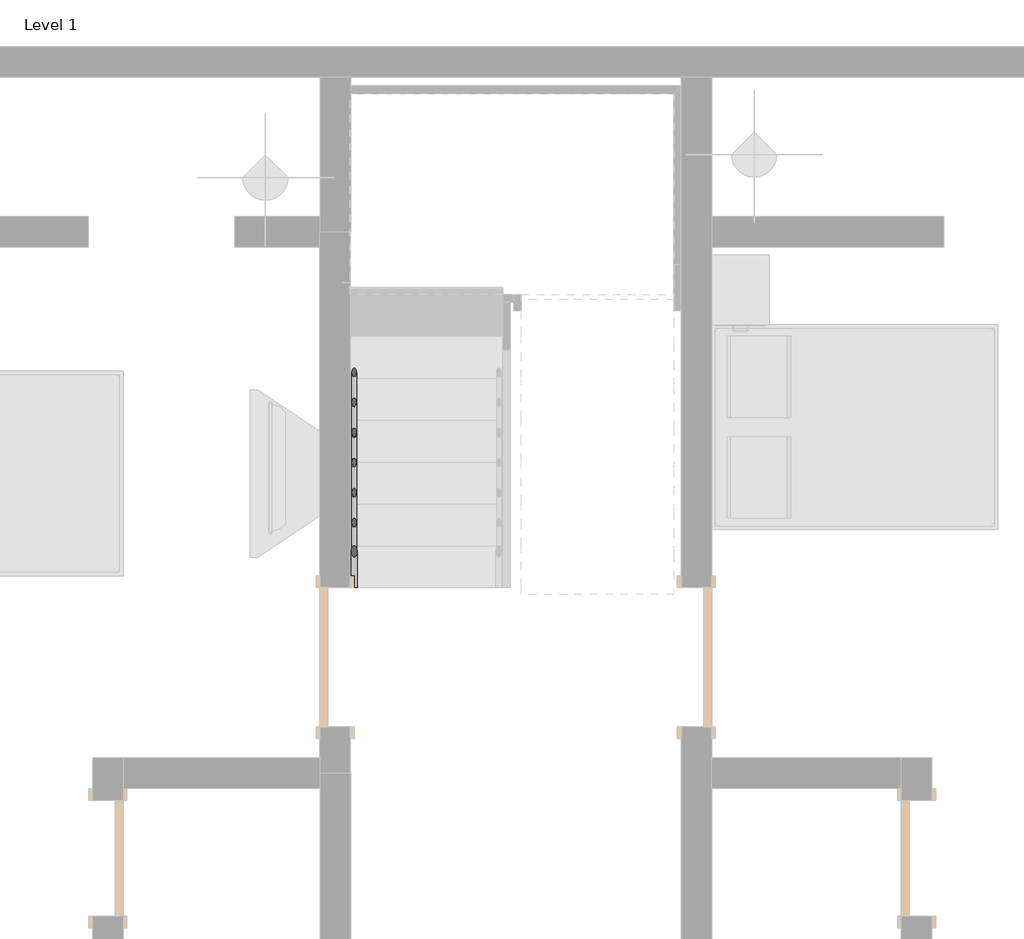
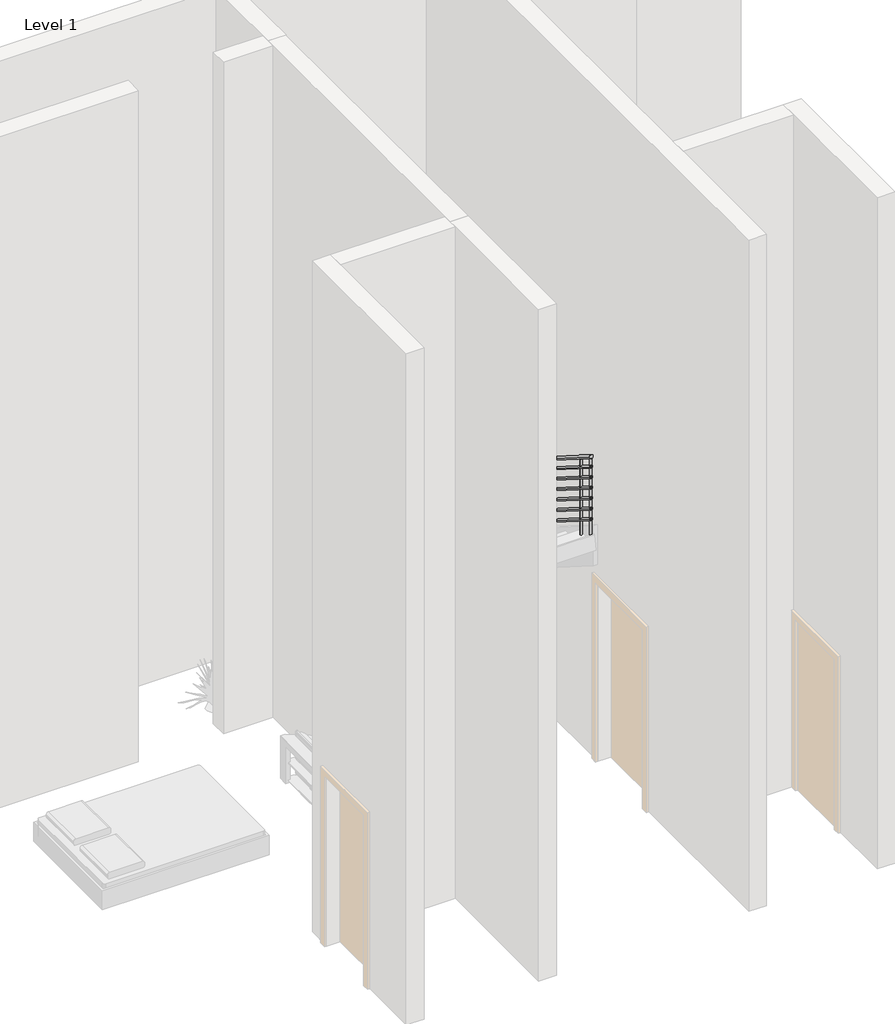
# One storey, part 3 of 4: 1 railing.
"""IFC4 building model written with IfcOpenShell, lengths in millimetres."""

from ifc_helpers import new_model, si_unit, point, frame, frame_2d, origin, place, context, project, spatial, circle_curve, ellipse_curve, trimmed, segment, composite_curve, outline, extrude, element, save
from ifc_brep_helpers import plane_surface, cylinder_surface, advanced_brep

model = new_model("IFC4")

# Units and contexts
model_context = context("Model", 3, world=origin())
ifc_project = project(units=[si_unit("LENGTHUNIT", "METRE", prefix="MILLI")], contexts=[model_context])

# Site, building, storey
site = spatial("IfcSite", under=ifc_project)
building = spatial("IfcBuilding", under=site)
storey = spatial("IfcBuildingStorey", under=building, Name="Level 1", Elevation=0.0)

# Railing
placement = place(None, origin())
element("IfcRailing", 1, ObjectType="900mm Pipe", at=placement, inside=storey, context=model_context, shape_type="SolidModel", body=[
    advanced_brep(
    [(-4517.5197318, 8898.7482221, 1050.2491997), (-4557.5197318, 8898.7482221, 1050.2491997), (-4517.5197318, 10829.5416751, 2271.3043478), (-4557.5197318, 10829.5416751, 2271.3043478), (-4517.5197318, 12099.1482221, 2271.3043478), (-4557.5197318, 12139.1482221, 2271.3043478), (-2485.6681693, 12099.1482221, 2271.3043478), (-2445.6681693, 12139.1482221, 2271.3043478), (-2485.6681693, 11092.9547691, 2271.3043478), (-2445.6681693, 11092.9547691, 2271.3043478), (-2485.6681693, 8898.7482221, 3658.9448519), (-2445.6681693, 8898.7482221, 3658.9448519)],
    [
        (0, 1, ellipse_curve(frame((-4537.5197318, 8898.7482221, 1050.2491997), z_axis=(0.0, -1.0, 0.0), x_axis=(0.0, 0.0, -1.0)), 23.6638438, 20.0)),
        (1, 0, ellipse_curve(frame((-4537.5197318, 8898.7482221, 1050.2491997), z_axis=(0.0, -1.0, 0.0), x_axis=(0.0, 0.0, -1.0)), 23.6638438, 20.0)),
        (0, 2),
        (2, 3, ellipse_curve(frame((-4537.5197318, 10829.5416751, 2271.3043478), z_axis=(0.0, -0.9605132043335073, -0.2782344053149759), x_axis=(0.0, 0.2782344053149766, -0.960513204333507)), 20.822202, 20.0)),
        (3, 1),
        (3, 2, ellipse_curve(frame((-4537.5197318, 10829.5416751, 2271.3043478), z_axis=(0.0, -0.9605132043335073, -0.2782344053149759), x_axis=(0.0, 0.2782344053149766, -0.960513204333507)), 20.822202, 20.0)),
        (2, 4),
        (4, 5, ellipse_curve(frame((-4537.5197318, 12119.1482221, 2271.3043478), z_axis=(-0.7071067811865482, -0.7071067811865468, 0.0), x_axis=(0.7071067811865468, -0.7071067811865482, 0.0)), 28.2842712, 20.0)),
        (5, 3),
        (5, 4, ellipse_curve(frame((-4537.5197318, 12119.1482221, 2271.3043478), z_axis=(-0.7071067811865482, -0.7071067811865468, 0.0), x_axis=(0.7071067811865468, -0.7071067811865482, 0.0)), 28.2842712, 20.0)),
        (4, 6),
        (6, 7, ellipse_curve(frame((-2465.6681693, 12119.1482221, 2271.3043478), z_axis=(-0.7071067811865469, 0.7071067811865481, 0.0), x_axis=(-0.7071067811865481, -0.7071067811865469, 0.0)), 28.2842712, 20.0)),
        (7, 5),
        (7, 6, ellipse_curve(frame((-2465.6681693, 12119.1482221, 2271.3043478), z_axis=(-0.7071067811865469, 0.7071067811865481, 0.0), x_axis=(-0.7071067811865481, -0.7071067811865469, 0.0)), 28.2842712, 20.0)),
        (6, 8),
        (8, 9, ellipse_curve(frame((-2465.6681693, 11092.9547691, 2271.3043478), z_axis=(0.0, 0.9605132043335073, -0.2782344053149755), x_axis=(0.0, 0.27823440531497573, 0.9605132043335072)), 20.822202, 20.0)),
        (9, 7),
        (9, 8, ellipse_curve(frame((-2465.6681693, 11092.9547691, 2271.3043478), z_axis=(0.0, 0.9605132043335073, -0.2782344053149755), x_axis=(0.0, 0.27823440531497573, 0.9605132043335072)), 20.822202, 20.0)),
        (10, 11, ellipse_curve(frame((-2465.6681693, 8898.7482221, 3658.9448519), z_axis=(0.0, -1.0, 0.0), x_axis=(0.0, 0.0, -1.0)), 23.6638438, 20.0)),
        (11, 10, ellipse_curve(frame((-2465.6681693, 8898.7482221, 3658.9448519), z_axis=(0.0, -1.0, 0.0), x_axis=(0.0, 0.0, -1.0)), 23.6638438, 20.0)),
        (8, 10),
        (11, 9),
    ],
    [
        plane_surface(frame((-4537.5197318, 8898.7482221, 1073.9130435), z_axis=(0.0, -1.0, 0.0), x_axis=(0.0, 0.0, 1.0))),
        cylinder_surface(frame((-4537.5197318, 8909.4381349, 1057.0096189), z_axis=(0.0, -0.8451712313980435, -0.5344956404098306), x_axis=(-1.0, 0.0, 0.0)), 20.0),
        cylinder_surface(frame((-4537.5197318, 10823.7482221, 2271.3043478), z_axis=(0.0, -1.0, 0.0), x_axis=(-1.0, 0.0, 0.0)), 20.0),
        cylinder_surface(frame((-4537.5197318, 12119.1482221, 2271.3043478), z_axis=(-1.0, 0.0, 0.0), x_axis=(0.0, 1.0, 0.0)), 20.0),
        cylinder_surface(frame((-2465.6681693, 12119.1482221, 2271.3043478), z_axis=(0.0, 1.0, 0.0), x_axis=(1.0, 0.0, 0.0)), 20.0),
        plane_surface(frame((-2465.6681693, 8898.7482221, 3682.6086957), z_axis=(0.0, -1.0, 0.0), x_axis=(0.0, 0.0, -1.0))),
        cylinder_surface(frame((-2465.6681693, 11088.0583093, 2274.4009232), z_axis=(0.0, 0.8451712313980438, -0.53449564040983), x_axis=(1.0, 0.0, 0.0)), 20.0),
    ],
    [
        (0, [[1, 2]]),
        (1, [[-1, 3, 4, 5]]),
        (1, [[-2, -5, 6, -3]]),
        (2, [[-4, 7, 8, 9]]),
        (2, [[-6, -9, 10, -7]]),
        (3, [[-8, 11, 12, 13]]),
        (3, [[-10, -13, 14, -11]]),
        (4, [[-12, 15, 16, 17]]),
        (4, [[-14, -17, 18, -15]]),
        (5, [[19, 20]]),
        (6, [[-16, 21, -20, 22]]),
        (6, [[-18, -22, -19, -21]]),
    ],
),
    advanced_brep(
    [(-4522.5197318, 8898.7482221, 931.1651606), (-4552.5197318, 8898.7482221, 931.1651606), (-4522.5197318, 10828.0933118, 2151.3043478), (-4552.5197318, 10828.0933118, 2151.3043478), (-4522.5197318, 12104.1482221, 2151.3043478), (-4552.5197318, 12134.1482221, 2151.3043478), (-2480.6681693, 12104.1482221, 2151.3043478), (-2450.6681693, 12134.1482221, 2151.3043478), (-2480.6681693, 11094.4031323, 2151.3043478), (-2450.6681693, 11094.4031323, 2151.3043478), (-2480.6681693, 8898.7482221, 3539.8608128), (-2450.6681693, 8898.7482221, 3539.8608128)],
    [
        (0, 1, ellipse_curve(frame((-4537.5197318, 8898.7482221, 931.1651606), z_axis=(0.0, -1.0, 0.0), x_axis=(0.0, 0.0, -1.0)), 17.7478828, 15.0)),
        (1, 0, ellipse_curve(frame((-4537.5197318, 8898.7482221, 931.1651606), z_axis=(0.0, -1.0, 0.0), x_axis=(0.0, 0.0, -1.0)), 17.7478828, 15.0)),
        (0, 2),
        (2, 3, ellipse_curve(frame((-4537.5197318, 10828.0933118, 2151.3043478), z_axis=(0.0, -0.9605132043335073, -0.2782344053149759), x_axis=(0.0, 0.2782344053149766, -0.960513204333507)), 15.6166515, 15.0)),
        (3, 1),
        (3, 2, ellipse_curve(frame((-4537.5197318, 10828.0933118, 2151.3043478), z_axis=(0.0, -0.9605132043335073, -0.2782344053149759), x_axis=(0.0, 0.2782344053149766, -0.960513204333507)), 15.6166515, 15.0)),
        (2, 4),
        (4, 5, ellipse_curve(frame((-4537.5197318, 12119.1482221, 2151.3043478), z_axis=(-0.7071067811865482, -0.7071067811865468, 0.0), x_axis=(0.7071067811865468, -0.7071067811865482, 0.0)), 21.2132034, 15.0)),
        (5, 3),
        (5, 4, ellipse_curve(frame((-4537.5197318, 12119.1482221, 2151.3043478), z_axis=(-0.7071067811865482, -0.7071067811865468, 0.0), x_axis=(0.7071067811865468, -0.7071067811865482, 0.0)), 21.2132034, 15.0)),
        (4, 6),
        (6, 7, ellipse_curve(frame((-2465.6681693, 12119.1482221, 2151.3043478), z_axis=(-0.7071067811865469, 0.7071067811865481, 0.0), x_axis=(-0.7071067811865481, -0.7071067811865469, 0.0)), 21.2132034, 15.0)),
        (7, 5),
        (7, 6, ellipse_curve(frame((-2465.6681693, 12119.1482221, 2151.3043478), z_axis=(-0.7071067811865469, 0.7071067811865481, 0.0), x_axis=(-0.7071067811865481, -0.7071067811865469, 0.0)), 21.2132034, 15.0)),
        (6, 8),
        (8, 9, ellipse_curve(frame((-2465.6681693, 11094.4031323, 2151.3043478), z_axis=(0.0, 0.9605132043335073, -0.27823440531497545), x_axis=(0.0, 0.2782344053149758, 0.9605132043335072)), 15.6166515, 15.0)),
        (9, 7),
        (9, 8, ellipse_curve(frame((-2465.6681693, 11094.4031323, 2151.3043478), z_axis=(0.0, 0.9605132043335073, -0.27823440531497545), x_axis=(0.0, 0.2782344053149758, 0.9605132043335072)), 15.6166515, 15.0)),
        (10, 11, ellipse_curve(frame((-2465.6681693, 8898.7482221, 3539.8608128), z_axis=(0.0, -1.0, 0.0), x_axis=(0.0, 0.0, -1.0)), 17.7478828, 15.0)),
        (11, 10, ellipse_curve(frame((-2465.6681693, 8898.7482221, 3539.8608128), z_axis=(0.0, -1.0, 0.0), x_axis=(0.0, 0.0, -1.0)), 17.7478828, 15.0)),
        (8, 10),
        (11, 9),
    ],
    [
        plane_surface(frame((-4537.5197318, 8898.7482221, 948.9130435), z_axis=(0.0, -1.0, 0.0), x_axis=(0.0, 0.0, 1.0))),
        cylinder_surface(frame((-4537.5197318, 8906.7656567, 936.235475), z_axis=(0.0, -0.8451712313980435, -0.5344956404098306), x_axis=(-1.0, 0.0, 0.0)), 15.0),
        cylinder_surface(frame((-4537.5197318, 10823.7482221, 2151.3043478), z_axis=(0.0, -1.0, 0.0), x_axis=(-1.0, 0.0, 0.0)), 15.0),
        cylinder_surface(frame((-4537.5197318, 12119.1482221, 2151.3043478), z_axis=(-1.0, 0.0, 0.0), x_axis=(0.0, 1.0, 0.0)), 15.0),
        cylinder_surface(frame((-2465.6681693, 12119.1482221, 2151.3043478), z_axis=(0.0, 1.0, 0.0), x_axis=(1.0, 0.0, 0.0)), 15.0),
        plane_surface(frame((-2465.6681693, 8898.7482221, 3557.6086957), z_axis=(0.0, -1.0, 0.0), x_axis=(0.0, 0.0, -1.0))),
        cylinder_surface(frame((-2465.6681693, 11090.7307875, 2153.6267794), z_axis=(0.0, 0.845171231398044, -0.5344956404098299), x_axis=(1.0, 0.0, 0.0)), 15.0),
    ],
    [
        (0, [[1, 2]]),
        (1, [[-1, 3, 4, 5]]),
        (1, [[-2, -5, 6, -3]]),
        (2, [[-4, 7, 8, 9]]),
        (2, [[-6, -9, 10, -7]]),
        (3, [[-8, 11, 12, 13]]),
        (3, [[-10, -13, 14, -11]]),
        (4, [[-12, 15, 16, 17]]),
        (4, [[-14, -17, 18, -15]]),
        (5, [[19, 20]]),
        (6, [[-16, 21, -20, 22]]),
        (6, [[-18, -22, -19, -21]]),
    ],
),
    advanced_brep(
    [(-4522.5197318, 8898.7482221, 806.1651606), (-4552.5197318, 8898.7482221, 806.1651606), (-4522.5197318, 10828.0933118, 2026.3043478), (-4552.5197318, 10828.0933118, 2026.3043478), (-4522.5197318, 12104.1482221, 2026.3043478), (-4552.5197318, 12134.1482221, 2026.3043478), (-2480.6681693, 12104.1482221, 2026.3043478), (-2450.6681693, 12134.1482221, 2026.3043478), (-2480.6681693, 11094.4031323, 2026.3043478), (-2450.6681693, 11094.4031323, 2026.3043478), (-2480.6681693, 8898.7482221, 3414.8608128), (-2450.6681693, 8898.7482221, 3414.8608128)],
    [
        (0, 1, ellipse_curve(frame((-4537.5197318, 8898.7482221, 806.1651606), z_axis=(0.0, -1.0, 0.0), x_axis=(0.0, 0.0, -1.0)), 17.7478828, 15.0)),
        (1, 0, ellipse_curve(frame((-4537.5197318, 8898.7482221, 806.1651606), z_axis=(0.0, -1.0, 0.0), x_axis=(0.0, 0.0, -1.0)), 17.7478828, 15.0)),
        (0, 2),
        (2, 3, ellipse_curve(frame((-4537.5197318, 10828.0933118, 2026.3043478), z_axis=(0.0, -0.9605132043335073, -0.2782344053149759), x_axis=(0.0, 0.2782344053149766, -0.960513204333507)), 15.6166515, 15.0)),
        (3, 1),
        (3, 2, ellipse_curve(frame((-4537.5197318, 10828.0933118, 2026.3043478), z_axis=(0.0, -0.9605132043335073, -0.2782344053149759), x_axis=(0.0, 0.2782344053149766, -0.960513204333507)), 15.6166515, 15.0)),
        (2, 4),
        (4, 5, ellipse_curve(frame((-4537.5197318, 12119.1482221, 2026.3043478), z_axis=(-0.7071067811865482, -0.7071067811865468, 0.0), x_axis=(0.7071067811865468, -0.7071067811865482, 0.0)), 21.2132034, 15.0)),
        (5, 3),
        (5, 4, ellipse_curve(frame((-4537.5197318, 12119.1482221, 2026.3043478), z_axis=(-0.7071067811865482, -0.7071067811865468, 0.0), x_axis=(0.7071067811865468, -0.7071067811865482, 0.0)), 21.2132034, 15.0)),
        (4, 6),
        (6, 7, ellipse_curve(frame((-2465.6681693, 12119.1482221, 2026.3043478), z_axis=(-0.7071067811865469, 0.7071067811865481, 0.0), x_axis=(-0.7071067811865481, -0.7071067811865469, 0.0)), 21.2132034, 15.0)),
        (7, 5),
        (7, 6, ellipse_curve(frame((-2465.6681693, 12119.1482221, 2026.3043478), z_axis=(-0.7071067811865469, 0.7071067811865481, 0.0), x_axis=(-0.7071067811865481, -0.7071067811865469, 0.0)), 21.2132034, 15.0)),
        (6, 8),
        (8, 9, ellipse_curve(frame((-2465.6681693, 11094.4031323, 2026.3043478), z_axis=(0.0, 0.9605132043335073, -0.2782344053149755), x_axis=(0.0, 0.27823440531497573, 0.9605132043335072)), 15.6166515, 15.0)),
        (9, 7),
        (9, 8, ellipse_curve(frame((-2465.6681693, 11094.4031323, 2026.3043478), z_axis=(0.0, 0.9605132043335073, -0.2782344053149755), x_axis=(0.0, 0.27823440531497573, 0.9605132043335072)), 15.6166515, 15.0)),
        (10, 11, ellipse_curve(frame((-2465.6681693, 8898.7482221, 3414.8608128), z_axis=(0.0, -1.0, 0.0), x_axis=(0.0, 0.0, -1.0)), 17.7478828, 15.0)),
        (11, 10, ellipse_curve(frame((-2465.6681693, 8898.7482221, 3414.8608128), z_axis=(0.0, -1.0, 0.0), x_axis=(0.0, 0.0, -1.0)), 17.7478828, 15.0)),
        (8, 10),
        (11, 9),
    ],
    [
        plane_surface(frame((-4537.5197318, 8898.7482221, 823.9130435), z_axis=(0.0, -1.0, 0.0), x_axis=(0.0, 0.0, 1.0))),
        cylinder_surface(frame((-4537.5197318, 8906.7656567, 811.235475), z_axis=(0.0, -0.8451712313980435, -0.5344956404098306), x_axis=(-1.0, 0.0, 0.0)), 15.0),
        cylinder_surface(frame((-4537.5197318, 10823.7482221, 2026.3043478), z_axis=(0.0, -1.0, 0.0), x_axis=(-1.0, 0.0, 0.0)), 15.0),
        cylinder_surface(frame((-4537.5197318, 12119.1482221, 2026.3043478), z_axis=(-1.0, 0.0, 0.0), x_axis=(0.0, 1.0, 0.0)), 15.0),
        cylinder_surface(frame((-2465.6681693, 12119.1482221, 2026.3043478), z_axis=(0.0, 1.0, 0.0), x_axis=(1.0, 0.0, 0.0)), 15.0),
        plane_surface(frame((-2465.6681693, 8898.7482221, 3432.6086957), z_axis=(0.0, -1.0, 0.0), x_axis=(0.0, 0.0, -1.0))),
        cylinder_surface(frame((-2465.6681693, 11090.7307875, 2028.6267794), z_axis=(0.0, 0.8451712313980438, -0.53449564040983), x_axis=(1.0, 0.0, 0.0)), 15.0),
    ],
    [
        (0, [[1, 2]]),
        (1, [[-1, 3, 4, 5]]),
        (1, [[-2, -5, 6, -3]]),
        (2, [[-4, 7, 8, 9]]),
        (2, [[-6, -9, 10, -7]]),
        (3, [[-8, 11, 12, 13]]),
        (3, [[-10, -13, 14, -11]]),
        (4, [[-12, 15, 16, 17]]),
        (4, [[-14, -17, 18, -15]]),
        (5, [[19, 20]]),
        (6, [[-16, 21, -20, 22]]),
        (6, [[-18, -22, -19, -21]]),
    ],
),
    advanced_brep(
    [(-4522.5197318, 8898.7482221, 681.1651606), (-4552.5197318, 8898.7482221, 681.1651606), (-4522.5197318, 10828.0933118, 1901.3043478), (-4552.5197318, 10828.0933118, 1901.3043478), (-4522.5197318, 12104.1482221, 1901.3043478), (-4552.5197318, 12134.1482221, 1901.3043478), (-2480.6681693, 12104.1482221, 1901.3043478), (-2450.6681693, 12134.1482221, 1901.3043478), (-2480.6681693, 11094.4031323, 1901.3043478), (-2450.6681693, 11094.4031323, 1901.3043478), (-2480.6681693, 8898.7482221, 3289.8608128), (-2450.6681693, 8898.7482221, 3289.8608128)],
    [
        (0, 1, ellipse_curve(frame((-4537.5197318, 8898.7482221, 681.1651606), z_axis=(0.0, -1.0, 0.0), x_axis=(0.0, 0.0, -1.0)), 17.7478828, 15.0)),
        (1, 0, ellipse_curve(frame((-4537.5197318, 8898.7482221, 681.1651606), z_axis=(0.0, -1.0, 0.0), x_axis=(0.0, 0.0, -1.0)), 17.7478828, 15.0)),
        (0, 2),
        (2, 3, ellipse_curve(frame((-4537.5197318, 10828.0933118, 1901.3043478), z_axis=(0.0, -0.9605132043335073, -0.2782344053149759), x_axis=(0.0, 0.2782344053149766, -0.960513204333507)), 15.6166515, 15.0)),
        (3, 1),
        (3, 2, ellipse_curve(frame((-4537.5197318, 10828.0933118, 1901.3043478), z_axis=(0.0, -0.9605132043335073, -0.2782344053149759), x_axis=(0.0, 0.2782344053149766, -0.960513204333507)), 15.6166515, 15.0)),
        (2, 4),
        (4, 5, ellipse_curve(frame((-4537.5197318, 12119.1482221, 1901.3043478), z_axis=(-0.7071067811865482, -0.7071067811865468, 0.0), x_axis=(0.7071067811865468, -0.7071067811865482, 0.0)), 21.2132034, 15.0)),
        (5, 3),
        (5, 4, ellipse_curve(frame((-4537.5197318, 12119.1482221, 1901.3043478), z_axis=(-0.7071067811865482, -0.7071067811865468, 0.0), x_axis=(0.7071067811865468, -0.7071067811865482, 0.0)), 21.2132034, 15.0)),
        (4, 6),
        (6, 7, ellipse_curve(frame((-2465.6681693, 12119.1482221, 1901.3043478), z_axis=(-0.7071067811865469, 0.7071067811865481, 0.0), x_axis=(-0.7071067811865481, -0.7071067811865469, 0.0)), 21.2132034, 15.0)),
        (7, 5),
        (7, 6, ellipse_curve(frame((-2465.6681693, 12119.1482221, 1901.3043478), z_axis=(-0.7071067811865469, 0.7071067811865481, 0.0), x_axis=(-0.7071067811865481, -0.7071067811865469, 0.0)), 21.2132034, 15.0)),
        (6, 8),
        (8, 9, ellipse_curve(frame((-2465.6681693, 11094.4031323, 1901.3043478), z_axis=(0.0, 0.9605132043335073, -0.27823440531497556), x_axis=(0.0, 0.2782344053149757, 0.9605132043335073)), 15.6166515, 15.0)),
        (9, 7),
        (9, 8, ellipse_curve(frame((-2465.6681693, 11094.4031323, 1901.3043478), z_axis=(0.0, 0.9605132043335073, -0.27823440531497556), x_axis=(0.0, 0.2782344053149757, 0.9605132043335073)), 15.6166515, 15.0)),
        (10, 11, ellipse_curve(frame((-2465.6681693, 8898.7482221, 3289.8608128), z_axis=(0.0, -1.0, 0.0), x_axis=(0.0, 0.0, -1.0)), 17.7478828, 15.0)),
        (11, 10, ellipse_curve(frame((-2465.6681693, 8898.7482221, 3289.8608128), z_axis=(0.0, -1.0, 0.0), x_axis=(0.0, 0.0, -1.0)), 17.7478828, 15.0)),
        (8, 10),
        (11, 9),
    ],
    [
        plane_surface(frame((-4537.5197318, 8898.7482221, 698.9130435), z_axis=(0.0, -1.0, 0.0), x_axis=(0.0, 0.0, 1.0))),
        cylinder_surface(frame((-4537.5197318, 8906.7656567, 686.235475), z_axis=(0.0, -0.8451712313980435, -0.5344956404098306), x_axis=(-1.0, 0.0, 0.0)), 15.0),
        cylinder_surface(frame((-4537.5197318, 10823.7482221, 1901.3043478), z_axis=(0.0, -1.0, 0.0), x_axis=(-1.0, 0.0, 0.0)), 15.0),
        cylinder_surface(frame((-4537.5197318, 12119.1482221, 1901.3043478), z_axis=(-1.0, 0.0, 0.0), x_axis=(0.0, 1.0, 0.0)), 15.0),
        cylinder_surface(frame((-2465.6681693, 12119.1482221, 1901.3043478), z_axis=(0.0, 1.0, 0.0), x_axis=(1.0, 0.0, 0.0)), 15.0),
        plane_surface(frame((-2465.6681693, 8898.7482221, 3307.6086957), z_axis=(0.0, -1.0, 0.0), x_axis=(0.0, 0.0, -1.0))),
        cylinder_surface(frame((-2465.6681693, 11090.7307875, 1903.6267794), z_axis=(0.0, 0.8451712313980438, -0.5344956404098301), x_axis=(1.0, 0.0, 0.0)), 15.0),
    ],
    [
        (0, [[1, 2]]),
        (1, [[-1, 3, 4, 5]]),
        (1, [[-2, -5, 6, -3]]),
        (2, [[-4, 7, 8, 9]]),
        (2, [[-6, -9, 10, -7]]),
        (3, [[-8, 11, 12, 13]]),
        (3, [[-10, -13, 14, -11]]),
        (4, [[-12, 15, 16, 17]]),
        (4, [[-14, -17, 18, -15]]),
        (5, [[19, 20]]),
        (6, [[-16, 21, -20, 22]]),
        (6, [[-18, -22, -19, -21]]),
    ],
),
    advanced_brep(
    [(-4522.5197318, 8898.7482221, 556.1651606), (-4552.5197318, 8898.7482221, 556.1651606), (-4522.5197318, 10828.0933118, 1776.3043478), (-4552.5197318, 10828.0933118, 1776.3043478), (-4522.5197318, 12104.1482221, 1776.3043478), (-4552.5197318, 12134.1482221, 1776.3043478), (-2480.6681693, 12104.1482221, 1776.3043478), (-2450.6681693, 12134.1482221, 1776.3043478), (-2480.6681693, 11094.4031323, 1776.3043478), (-2450.6681693, 11094.4031323, 1776.3043478), (-2480.6681693, 8898.7482221, 3164.8608128), (-2450.6681693, 8898.7482221, 3164.8608128)],
    [
        (0, 1, ellipse_curve(frame((-4537.5197318, 8898.7482221, 556.1651606), z_axis=(0.0, -1.0, 0.0), x_axis=(0.0, 0.0, -1.0)), 17.7478828, 15.0)),
        (1, 0, ellipse_curve(frame((-4537.5197318, 8898.7482221, 556.1651606), z_axis=(0.0, -1.0, 0.0), x_axis=(0.0, 0.0, -1.0)), 17.7478828, 15.0)),
        (0, 2),
        (2, 3, ellipse_curve(frame((-4537.5197318, 10828.0933118, 1776.3043478), z_axis=(0.0, -0.9605132043335073, -0.2782344053149759), x_axis=(0.0, 0.2782344053149766, -0.960513204333507)), 15.6166515, 15.0)),
        (3, 1),
        (3, 2, ellipse_curve(frame((-4537.5197318, 10828.0933118, 1776.3043478), z_axis=(0.0, -0.9605132043335073, -0.2782344053149759), x_axis=(0.0, 0.2782344053149766, -0.960513204333507)), 15.6166515, 15.0)),
        (2, 4),
        (4, 5, ellipse_curve(frame((-4537.5197318, 12119.1482221, 1776.3043478), z_axis=(-0.7071067811865482, -0.7071067811865468, 0.0), x_axis=(0.7071067811865468, -0.7071067811865482, 0.0)), 21.2132034, 15.0)),
        (5, 3),
        (5, 4, ellipse_curve(frame((-4537.5197318, 12119.1482221, 1776.3043478), z_axis=(-0.7071067811865482, -0.7071067811865468, 0.0), x_axis=(0.7071067811865468, -0.7071067811865482, 0.0)), 21.2132034, 15.0)),
        (4, 6),
        (6, 7, ellipse_curve(frame((-2465.6681693, 12119.1482221, 1776.3043478), z_axis=(-0.7071067811865469, 0.7071067811865481, 0.0), x_axis=(-0.7071067811865481, -0.7071067811865469, 0.0)), 21.2132034, 15.0)),
        (7, 5),
        (7, 6, ellipse_curve(frame((-2465.6681693, 12119.1482221, 1776.3043478), z_axis=(-0.7071067811865469, 0.7071067811865481, 0.0), x_axis=(-0.7071067811865481, -0.7071067811865469, 0.0)), 21.2132034, 15.0)),
        (6, 8),
        (8, 9, ellipse_curve(frame((-2465.6681693, 11094.4031323, 1776.3043478), z_axis=(0.0, 0.9605132043335073, -0.2782344053149755), x_axis=(0.0, 0.27823440531497573, 0.9605132043335072)), 15.6166515, 15.0)),
        (9, 7),
        (9, 8, ellipse_curve(frame((-2465.6681693, 11094.4031323, 1776.3043478), z_axis=(0.0, 0.9605132043335073, -0.2782344053149755), x_axis=(0.0, 0.27823440531497573, 0.9605132043335072)), 15.6166515, 15.0)),
        (10, 11, ellipse_curve(frame((-2465.6681693, 8898.7482221, 3164.8608128), z_axis=(0.0, -1.0, 0.0), x_axis=(0.0, 0.0, -1.0)), 17.7478828, 15.0)),
        (11, 10, ellipse_curve(frame((-2465.6681693, 8898.7482221, 3164.8608128), z_axis=(0.0, -1.0, 0.0), x_axis=(0.0, 0.0, -1.0)), 17.7478828, 15.0)),
        (8, 10),
        (11, 9),
    ],
    [
        plane_surface(frame((-4537.5197318, 8898.7482221, 573.9130435), z_axis=(0.0, -1.0, 0.0), x_axis=(0.0, 0.0, 1.0))),
        cylinder_surface(frame((-4537.5197318, 8906.7656567, 561.235475), z_axis=(0.0, -0.8451712313980435, -0.5344956404098306), x_axis=(-1.0, 0.0, 0.0)), 15.0),
        cylinder_surface(frame((-4537.5197318, 10823.7482221, 1776.3043478), z_axis=(0.0, -1.0, 0.0), x_axis=(-1.0, 0.0, 0.0)), 15.0),
        cylinder_surface(frame((-4537.5197318, 12119.1482221, 1776.3043478), z_axis=(-1.0, 0.0, 0.0), x_axis=(0.0, 1.0, 0.0)), 15.0),
        cylinder_surface(frame((-2465.6681693, 12119.1482221, 1776.3043478), z_axis=(0.0, 1.0, 0.0), x_axis=(1.0, 0.0, 0.0)), 15.0),
        plane_surface(frame((-2465.6681693, 8898.7482221, 3182.6086957), z_axis=(0.0, -1.0, 0.0), x_axis=(0.0, 0.0, -1.0))),
        cylinder_surface(frame((-2465.6681693, 11090.7307875, 1778.6267794), z_axis=(0.0, 0.8451712313980438, -0.53449564040983), x_axis=(1.0, 0.0, 0.0)), 15.0),
    ],
    [
        (0, [[1, 2]]),
        (1, [[-1, 3, 4, 5]]),
        (1, [[-2, -5, 6, -3]]),
        (2, [[-4, 7, 8, 9]]),
        (2, [[-6, -9, 10, -7]]),
        (3, [[-8, 11, 12, 13]]),
        (3, [[-10, -13, 14, -11]]),
        (4, [[-12, 15, 16, 17]]),
        (4, [[-14, -17, 18, -15]]),
        (5, [[19, 20]]),
        (6, [[-16, 21, -20, 22]]),
        (6, [[-18, -22, -19, -21]]),
    ],
),
    advanced_brep(
    [(-4522.5197318, 8898.7482221, 431.1651606), (-4552.5197318, 8898.7482221, 431.1651606), (-4522.5197318, 10828.0933118, 1651.3043478), (-4552.5197318, 10828.0933118, 1651.3043478), (-4522.5197318, 12104.1482221, 1651.3043478), (-4552.5197318, 12134.1482221, 1651.3043478), (-2480.6681693, 12104.1482221, 1651.3043478), (-2450.6681693, 12134.1482221, 1651.3043478), (-2480.6681693, 11094.4031323, 1651.3043478), (-2450.6681693, 11094.4031323, 1651.3043478), (-2480.6681693, 8898.7482221, 3039.8608128), (-2450.6681693, 8898.7482221, 3039.8608128)],
    [
        (0, 1, ellipse_curve(frame((-4537.5197318, 8898.7482221, 431.1651606), z_axis=(0.0, -1.0, 0.0), x_axis=(0.0, 0.0, -1.0)), 17.7478828, 15.0)),
        (1, 0, ellipse_curve(frame((-4537.5197318, 8898.7482221, 431.1651606), z_axis=(0.0, -1.0, 0.0), x_axis=(0.0, 0.0, -1.0)), 17.7478828, 15.0)),
        (0, 2),
        (2, 3, ellipse_curve(frame((-4537.5197318, 10828.0933118, 1651.3043478), z_axis=(0.0, -0.9605132043335073, -0.2782344053149759), x_axis=(0.0, 0.2782344053149766, -0.960513204333507)), 15.6166515, 15.0)),
        (3, 1),
        (3, 2, ellipse_curve(frame((-4537.5197318, 10828.0933118, 1651.3043478), z_axis=(0.0, -0.9605132043335073, -0.2782344053149759), x_axis=(0.0, 0.2782344053149766, -0.960513204333507)), 15.6166515, 15.0)),
        (2, 4),
        (4, 5, ellipse_curve(frame((-4537.5197318, 12119.1482221, 1651.3043478), z_axis=(-0.7071067811865482, -0.7071067811865468, 0.0), x_axis=(0.7071067811865468, -0.7071067811865482, 0.0)), 21.2132034, 15.0)),
        (5, 3),
        (5, 4, ellipse_curve(frame((-4537.5197318, 12119.1482221, 1651.3043478), z_axis=(-0.7071067811865482, -0.7071067811865468, 0.0), x_axis=(0.7071067811865468, -0.7071067811865482, 0.0)), 21.2132034, 15.0)),
        (4, 6),
        (6, 7, ellipse_curve(frame((-2465.6681693, 12119.1482221, 1651.3043478), z_axis=(-0.7071067811865469, 0.7071067811865481, 0.0), x_axis=(-0.7071067811865481, -0.7071067811865469, 0.0)), 21.2132034, 15.0)),
        (7, 5),
        (7, 6, ellipse_curve(frame((-2465.6681693, 12119.1482221, 1651.3043478), z_axis=(-0.7071067811865469, 0.7071067811865481, 0.0), x_axis=(-0.7071067811865481, -0.7071067811865469, 0.0)), 21.2132034, 15.0)),
        (6, 8),
        (8, 9, ellipse_curve(frame((-2465.6681693, 11094.4031323, 1651.3043478), z_axis=(0.0, 0.9605132043335073, -0.27823440531497545), x_axis=(0.0, 0.2782344053149758, 0.9605132043335072)), 15.6166515, 15.0)),
        (9, 7),
        (9, 8, ellipse_curve(frame((-2465.6681693, 11094.4031323, 1651.3043478), z_axis=(0.0, 0.9605132043335073, -0.27823440531497545), x_axis=(0.0, 0.2782344053149758, 0.9605132043335072)), 15.6166515, 15.0)),
        (10, 11, ellipse_curve(frame((-2465.6681693, 8898.7482221, 3039.8608128), z_axis=(0.0, -1.0, 0.0), x_axis=(0.0, 0.0, -1.0)), 17.7478828, 15.0)),
        (11, 10, ellipse_curve(frame((-2465.6681693, 8898.7482221, 3039.8608128), z_axis=(0.0, -1.0, 0.0), x_axis=(0.0, 0.0, -1.0)), 17.7478828, 15.0)),
        (8, 10),
        (11, 9),
    ],
    [
        plane_surface(frame((-4537.5197318, 8898.7482221, 448.9130435), z_axis=(0.0, -1.0, 0.0), x_axis=(0.0, 0.0, 1.0))),
        cylinder_surface(frame((-4537.5197318, 8906.7656567, 436.235475), z_axis=(0.0, -0.8451712313980435, -0.5344956404098306), x_axis=(-1.0, 0.0, 0.0)), 15.0),
        cylinder_surface(frame((-4537.5197318, 10823.7482221, 1651.3043478), z_axis=(0.0, -1.0, 0.0), x_axis=(-1.0, 0.0, 0.0)), 15.0),
        cylinder_surface(frame((-4537.5197318, 12119.1482221, 1651.3043478), z_axis=(-1.0, 0.0, 0.0), x_axis=(0.0, 1.0, 0.0)), 15.0),
        cylinder_surface(frame((-2465.6681693, 12119.1482221, 1651.3043478), z_axis=(0.0, 1.0, 0.0), x_axis=(1.0, 0.0, 0.0)), 15.0),
        plane_surface(frame((-2465.6681693, 8898.7482221, 3057.6086957), z_axis=(0.0, -1.0, 0.0), x_axis=(0.0, 0.0, -1.0))),
        cylinder_surface(frame((-2465.6681693, 11090.7307875, 1653.6267794), z_axis=(0.0, 0.845171231398044, -0.5344956404098299), x_axis=(1.0, 0.0, 0.0)), 15.0),
    ],
    [
        (0, [[1, 2]]),
        (1, [[-1, 3, 4, 5]]),
        (1, [[-2, -5, 6, -3]]),
        (2, [[-4, 7, 8, 9]]),
        (2, [[-6, -9, 10, -7]]),
        (3, [[-8, 11, 12, 13]]),
        (3, [[-10, -13, 14, -11]]),
        (4, [[-12, 15, 16, 17]]),
        (4, [[-14, -17, 18, -15]]),
        (5, [[19, 20]]),
        (6, [[-16, 21, -20, 22]]),
        (6, [[-18, -22, -19, -21]]),
    ],
),
    advanced_brep(
    [(-4522.5197318, 8898.7482221, 306.1651606), (-4552.5197318, 8898.7482221, 306.1651606), (-4522.5197318, 10828.0933118, 1526.3043478), (-4552.5197318, 10828.0933118, 1526.3043478), (-4522.5197318, 12104.1482221, 1526.3043478), (-4552.5197318, 12134.1482221, 1526.3043478), (-2480.6681693, 12104.1482221, 1526.3043478), (-2450.6681693, 12134.1482221, 1526.3043478), (-2480.6681693, 11094.4031323, 1526.3043478), (-2450.6681693, 11094.4031323, 1526.3043478), (-2480.6681693, 8898.7482221, 2914.8608128), (-2450.6681693, 8898.7482221, 2914.8608128)],
    [
        (0, 1, ellipse_curve(frame((-4537.5197318, 8898.7482221, 306.1651606), z_axis=(0.0, -1.0, 0.0), x_axis=(0.0, 0.0, -1.0)), 17.7478828, 15.0)),
        (1, 0, ellipse_curve(frame((-4537.5197318, 8898.7482221, 306.1651606), z_axis=(0.0, -1.0, 0.0), x_axis=(0.0, 0.0, -1.0)), 17.7478828, 15.0)),
        (0, 2),
        (2, 3, ellipse_curve(frame((-4537.5197318, 10828.0933118, 1526.3043478), z_axis=(0.0, -0.9605132043335073, -0.2782344053149759), x_axis=(0.0, 0.2782344053149766, -0.960513204333507)), 15.6166515, 15.0)),
        (3, 1),
        (3, 2, ellipse_curve(frame((-4537.5197318, 10828.0933118, 1526.3043478), z_axis=(0.0, -0.9605132043335073, -0.2782344053149759), x_axis=(0.0, 0.2782344053149766, -0.960513204333507)), 15.6166515, 15.0)),
        (2, 4),
        (4, 5, ellipse_curve(frame((-4537.5197318, 12119.1482221, 1526.3043478), z_axis=(-0.7071067811865482, -0.7071067811865468, 0.0), x_axis=(0.7071067811865468, -0.7071067811865482, 0.0)), 21.2132034, 15.0)),
        (5, 3),
        (5, 4, ellipse_curve(frame((-4537.5197318, 12119.1482221, 1526.3043478), z_axis=(-0.7071067811865482, -0.7071067811865468, 0.0), x_axis=(0.7071067811865468, -0.7071067811865482, 0.0)), 21.2132034, 15.0)),
        (4, 6),
        (6, 7, ellipse_curve(frame((-2465.6681693, 12119.1482221, 1526.3043478), z_axis=(-0.7071067811865469, 0.7071067811865481, 0.0), x_axis=(-0.7071067811865481, -0.7071067811865469, 0.0)), 21.2132034, 15.0)),
        (7, 5),
        (7, 6, ellipse_curve(frame((-2465.6681693, 12119.1482221, 1526.3043478), z_axis=(-0.7071067811865469, 0.7071067811865481, 0.0), x_axis=(-0.7071067811865481, -0.7071067811865469, 0.0)), 21.2132034, 15.0)),
        (6, 8),
        (8, 9, ellipse_curve(frame((-2465.6681693, 11094.4031323, 1526.3043478), z_axis=(0.0, 0.9605132043335073, -0.2782344053149755), x_axis=(0.0, 0.27823440531497573, 0.9605132043335072)), 15.6166515, 15.0)),
        (9, 7),
        (9, 8, ellipse_curve(frame((-2465.6681693, 11094.4031323, 1526.3043478), z_axis=(0.0, 0.9605132043335073, -0.2782344053149755), x_axis=(0.0, 0.27823440531497573, 0.9605132043335072)), 15.6166515, 15.0)),
        (10, 11, ellipse_curve(frame((-2465.6681693, 8898.7482221, 2914.8608128), z_axis=(0.0, -1.0, 0.0), x_axis=(0.0, 0.0, -1.0)), 17.7478828, 15.0)),
        (11, 10, ellipse_curve(frame((-2465.6681693, 8898.7482221, 2914.8608128), z_axis=(0.0, -1.0, 0.0), x_axis=(0.0, 0.0, -1.0)), 17.7478828, 15.0)),
        (8, 10),
        (11, 9),
    ],
    [
        plane_surface(frame((-4537.5197318, 8898.7482221, 323.9130435), z_axis=(0.0, -1.0, 0.0), x_axis=(0.0, 0.0, 1.0))),
        cylinder_surface(frame((-4537.5197318, 8906.7656567, 311.235475), z_axis=(0.0, -0.8451712313980435, -0.5344956404098306), x_axis=(-1.0, 0.0, 0.0)), 15.0),
        cylinder_surface(frame((-4537.5197318, 10823.7482221, 1526.3043478), z_axis=(0.0, -1.0, 0.0), x_axis=(-1.0, 0.0, 0.0)), 15.0),
        cylinder_surface(frame((-4537.5197318, 12119.1482221, 1526.3043478), z_axis=(-1.0, 0.0, 0.0), x_axis=(0.0, 1.0, 0.0)), 15.0),
        cylinder_surface(frame((-2465.6681693, 12119.1482221, 1526.3043478), z_axis=(0.0, 1.0, 0.0), x_axis=(1.0, 0.0, 0.0)), 15.0),
        plane_surface(frame((-2465.6681693, 8898.7482221, 2932.6086957), z_axis=(0.0, -1.0, 0.0), x_axis=(0.0, 0.0, -1.0))),
        cylinder_surface(frame((-2465.6681693, 11090.7307875, 1528.6267794), z_axis=(0.0, 0.8451712313980438, -0.53449564040983), x_axis=(1.0, 0.0, 0.0)), 15.0),
    ],
    [
        (0, [[1, 2]]),
        (1, [[-1, 3, 4, 5]]),
        (1, [[-2, -5, 6, -3]]),
        (2, [[-4, 7, 8, 9]]),
        (2, [[-6, -9, 10, -7]]),
        (3, [[-8, 11, 12, 13]]),
        (3, [[-10, -13, 14, -11]]),
        (4, [[-12, 15, 16, 17]]),
        (4, [[-14, -17, 18, -15]]),
        (5, [[19, 20]]),
        (6, [[-16, 21, -20, 22]]),
        (6, [[-18, -22, -19, -21]]),
    ],
),
    advanced_brep(
    [(-2453.1681693, 9098.7482221, 3508.7987946), (-2478.1681693, 9098.7482221, 3508.7987946), (-2478.1681693, 9098.7482221, 2608.6956522), (-2453.1681693, 9098.7482221, 2608.6956522)],
    [
        (0, 1, ellipse_curve(frame((-2465.6681693, 9098.7482221, 3508.7987946), z_axis=(0.0, -0.5344956404098302, -0.8451712313980437), x_axis=(0.0, -0.8451712313980437, 0.53449564040983)), 14.7899024, 12.5)),
        (1, 2),
        (2, 3, circle_curve(frame((-2465.6681693, 9098.7482221, 2608.6956522), z_axis=(0.0, 0.0, 1.0), x_axis=(-1.0, 0.0, 0.0)), 12.5)),
        (3, 0),
        (3, 2, circle_curve(frame((-2465.6681693, 9098.7482221, 2608.6956522), z_axis=(0.0, 0.0, 1.0), x_axis=(-1.0, 0.0, 0.0)), 12.5)),
        (1, 0, ellipse_curve(frame((-2465.6681693, 9098.7482221, 3508.7987946), z_axis=(0.0, -0.5344956404098302, -0.8451712313980437), x_axis=(0.0, -0.8451712313980437, 0.53449564040983)), 14.7899024, 12.5)),
    ],
    [
        cylinder_surface(frame((-2465.6681693, 9098.7482221, 2508.6956522), z_axis=(0.0, 0.0, 1.0), x_axis=(-1.0, 0.0, 0.0)), 12.5),
        plane_surface(frame((-2490.6681693, 9073.7482221, 3524.6090713), z_axis=(0.0, 0.5344956404098302, 0.8451712313980437), x_axis=(1.0, 0.0, 0.0))),
        plane_surface(frame((-2490.6681693, 9123.7482221, 2608.6956522), z_axis=(0.0, 0.0, -1.0), x_axis=(1.0, 0.0, 0.0))),
    ],
    [
        (0, [[1, 2, 3, 4]]),
        (0, [[5, -2, 6, -4]]),
        (1, [[-6, -1]]),
        (2, [[-5, -3]]),
    ],
),
    advanced_brep(
    [(-2453.1681693, 10098.7482221, 2876.3877274), (-2478.1681693, 10098.7482221, 2876.3877274), (-2478.1681693, 10098.7482221, 1913.0434783), (-2453.1681693, 10098.7482221, 1913.0434783)],
    [
        (0, 1, ellipse_curve(frame((-2465.6681693, 10098.7482221, 2876.3877274), z_axis=(0.0, -0.5344956404098302, -0.8451712313980437), x_axis=(0.0, -0.8451712313980437, 0.53449564040983)), 14.7899024, 12.5)),
        (1, 2),
        (2, 3, circle_curve(frame((-2465.6681693, 10098.7482221, 1913.0434783), z_axis=(0.0, 0.0, 1.0), x_axis=(-1.0, 0.0, 0.0)), 12.5)),
        (3, 0),
        (3, 2, circle_curve(frame((-2465.6681693, 10098.7482221, 1913.0434783), z_axis=(0.0, 0.0, 1.0), x_axis=(-1.0, 0.0, 0.0)), 12.5)),
        (1, 0, ellipse_curve(frame((-2465.6681693, 10098.7482221, 2876.3877274), z_axis=(0.0, -0.5344956404098302, -0.8451712313980437), x_axis=(0.0, -0.8451712313980437, 0.53449564040983)), 14.7899024, 12.5)),
    ],
    [
        cylinder_surface(frame((-2465.6681693, 10098.7482221, 1813.0434783), z_axis=(0.0, 0.0, 1.0), x_axis=(-1.0, 0.0, 0.0)), 12.5),
        plane_surface(frame((-2490.6681693, 10073.7482221, 2892.1980041), z_axis=(0.0, 0.5344956404098302, 0.8451712313980437), x_axis=(1.0, 0.0, 0.0))),
        plane_surface(frame((-2490.6681693, 10123.7482221, 1913.0434783), z_axis=(0.0, 0.0, -1.0), x_axis=(1.0, 0.0, 0.0))),
    ],
    [
        (0, [[1, 2, 3, 4]]),
        (0, [[5, -2, 6, -4]]),
        (1, [[-6, -1]]),
        (2, [[-5, -3]]),
    ],
),
    extrude(outline(composite_curve([segment(trimmed(circle_curve(frame_2d((-2465.6681693, 11119.1482221)), 12.5), [point((-2478.1681693, 11119.1482221))], [point((-2453.1681693, 11119.1482221))], False, "CARTESIAN"), True, "CONTINUOUS"), segment(trimmed(circle_curve(frame_2d((-2465.6681693, 11119.1482221)), 12.5), [point((-2453.1681693, 11119.1482221))], [point((-2478.1681693, 11119.1482221))], False, "CARTESIAN"), True, "CONTINUOUS")], self_intersect=False)), frame((0.0, 0.0, 1391.3043478), z_axis=(0.0, 0.0, 1.0), x_axis=(1.0, 0.0, 0.0)), (0.0, 0.0, 1.0), 860.0),
    extrude(outline(composite_curve([segment(trimmed(circle_curve(frame_2d((-2537.5197318, 12119.1482221)), 12.5), [point((-2537.5197318, 12106.6482221))], [point((-2537.5197318, 12131.6482221))], False, "CARTESIAN"), True, "CONTINUOUS"), segment(trimmed(circle_curve(frame_2d((-2537.5197318, 12119.1482221)), 12.5), [point((-2537.5197318, 12131.6482221))], [point((-2537.5197318, 12106.6482221))], False, "CARTESIAN"), True, "CONTINUOUS")], self_intersect=False)), frame((0.0, 0.0, 1391.3043478), z_axis=(0.0, 0.0, 1.0), x_axis=(1.0, 0.0, 0.0)), (0.0, 0.0, 1.0), 860.0),
    extrude(outline(composite_curve([segment(trimmed(circle_curve(frame_2d((-3537.5197318, 12119.1482221)), 12.5), [point((-3537.5197318, 12106.6482221))], [point((-3537.5197318, 12131.6482221))], False, "CARTESIAN"), True, "CONTINUOUS"), segment(trimmed(circle_curve(frame_2d((-3537.5197318, 12119.1482221)), 12.5), [point((-3537.5197318, 12131.6482221))], [point((-3537.5197318, 12106.6482221))], False, "CARTESIAN"), True, "CONTINUOUS")], self_intersect=False)), frame((0.0, 0.0, 1391.3043478), z_axis=(0.0, 0.0, 1.0), x_axis=(1.0, 0.0, 0.0)), (0.0, 0.0, 1.0), 860.0),
    extrude(outline(composite_curve([segment(trimmed(circle_curve(frame_2d((-4537.5197318, 11823.7482221)), 12.5), [point((-4525.0197318, 11823.7482221))], [point((-4550.0197318, 11823.7482221))], False, "CARTESIAN"), True, "CONTINUOUS"), segment(trimmed(circle_curve(frame_2d((-4537.5197318, 11823.7482221)), 12.5), [point((-4550.0197318, 11823.7482221))], [point((-4525.0197318, 11823.7482221))], False, "CARTESIAN"), True, "CONTINUOUS")], self_intersect=False)), frame((0.0, 0.0, 1391.3043478), z_axis=(0.0, 0.0, 1.0), x_axis=(1.0, 0.0, 0.0)), (0.0, 0.0, 1.0), 860.0),
    advanced_brep(
    [(-4550.0197318, 9898.7482221, 1658.9964231), (-4525.0197318, 9898.7482221, 1658.9964231), (-4525.0197318, 9898.7482221, 695.6521739), (-4550.0197318, 9898.7482221, 695.6521739)],
    [
        (0, 1, ellipse_curve(frame((-4537.5197318, 9898.7482221, 1658.9964231), z_axis=(0.0, 0.5344956404098302, -0.8451712313980437), x_axis=(0.0, 0.8451712313980437, 0.53449564040983)), 14.7899024, 12.5)),
        (1, 2),
        (2, 3, circle_curve(frame((-4537.5197318, 9898.7482221, 695.6521739), z_axis=(0.0, 0.0, 1.0), x_axis=(1.0, 0.0, 0.0)), 12.5)),
        (3, 0),
        (3, 2, circle_curve(frame((-4537.5197318, 9898.7482221, 695.6521739), z_axis=(0.0, 0.0, 1.0), x_axis=(1.0, 0.0, 0.0)), 12.5)),
        (1, 0, ellipse_curve(frame((-4537.5197318, 9898.7482221, 1658.9964231), z_axis=(0.0, 0.5344956404098302, -0.8451712313980437), x_axis=(0.0, 0.8451712313980437, 0.53449564040983)), 14.7899024, 12.5)),
    ],
    [
        cylinder_surface(frame((-4537.5197318, 9898.7482221, 595.6521739), z_axis=(0.0, 0.0, 1.0), x_axis=(1.0, 0.0, 0.0)), 12.5),
        plane_surface(frame((-4512.5197318, 9923.7482221, 1674.8066998), z_axis=(0.0, -0.5344956404098302, 0.8451712313980437), x_axis=(-1.0, 0.0, 0.0))),
        plane_surface(frame((-4512.5197318, 9873.7482221, 695.6521739), z_axis=(0.0, 0.0, -1.0), x_axis=(-1.0, 0.0, 0.0))),
    ],
    [
        (0, [[1, 2, 3, 4]]),
        (0, [[5, -2, 6, -4]]),
        (1, [[-6, -1]]),
        (2, [[-5, -3]]),
    ],
),
    extrude(outline(composite_curve([segment(trimmed(circle_curve(frame_2d((-2465.6681693, 11098.7482221)), 12.5), [point((-2478.1681693, 11098.7482221))], [point((-2453.1681693, 11098.7482221))], False, "CARTESIAN"), True, "CONTINUOUS"), segment(trimmed(circle_curve(frame_2d((-2465.6681693, 11098.7482221)), 12.5), [point((-2453.1681693, 11098.7482221))], [point((-2478.1681693, 11098.7482221))], False, "CARTESIAN"), True, "CONTINUOUS")], self_intersect=False)), frame((0.0, 0.0, 1391.3043478), z_axis=(0.0, 0.0, 1.0), x_axis=(1.0, 0.0, 0.0)), (0.0, 0.0, 1.0), 860.0),
    extrude(outline(composite_curve([segment(trimmed(circle_curve(frame_2d((-2465.6681693, 12119.1482221)), 12.5), [point((-2465.6681693, 12106.6482221))], [point((-2465.6681693, 12131.6482221))], False, "CARTESIAN"), True, "CONTINUOUS"), segment(trimmed(circle_curve(frame_2d((-2465.6681693, 12119.1482221)), 12.5), [point((-2465.6681693, 12131.6482221))], [point((-2465.6681693, 12106.6482221))], False, "CARTESIAN"), True, "CONTINUOUS")], self_intersect=False)), frame((0.0, 0.0, 1391.3043478), z_axis=(0.0, 0.0, 1.0), x_axis=(1.0, 0.0, 0.0)), (0.0, 0.0, 1.0), 860.0),
    extrude(outline(composite_curve([segment(trimmed(circle_curve(frame_2d((-4537.5197318, 12119.1482221)), 12.5), [point((-4525.0197318, 12119.1482221))], [point((-4550.0197318, 12119.1482221))], False, "CARTESIAN"), True, "CONTINUOUS"), segment(trimmed(circle_curve(frame_2d((-4537.5197318, 12119.1482221)), 12.5), [point((-4550.0197318, 12119.1482221))], [point((-4525.0197318, 12119.1482221))], False, "CARTESIAN"), True, "CONTINUOUS")], self_intersect=False)), frame((0.0, 0.0, 1391.3043478), z_axis=(0.0, 0.0, 1.0), x_axis=(1.0, 0.0, 0.0)), (0.0, 0.0, 1.0), 860.0),
    advanced_brep(
    [(-4550.0197318, 10823.7482221, 2243.9766602), (-4525.0197318, 10823.7482221, 2243.9766602), (-4525.0197318, 10823.7482221, 1391.3043478), (-4550.0197318, 10823.7482221, 1391.3043478)],
    [
        (0, 1, ellipse_curve(frame((-4537.5197318, 10823.7482221, 2243.9766602), z_axis=(0.0, 0.5344956404098302, -0.8451712313980437), x_axis=(0.0, 0.8451712313980437, 0.53449564040983)), 14.7899024, 12.5)),
        (1, 2),
        (2, 3, circle_curve(frame((-4537.5197318, 10823.7482221, 1391.3043478), z_axis=(0.0, 0.0, 1.0), x_axis=(1.0, 0.0, 0.0)), 12.5)),
        (3, 0),
        (3, 2, circle_curve(frame((-4537.5197318, 10823.7482221, 1391.3043478), z_axis=(0.0, 0.0, 1.0), x_axis=(1.0, 0.0, 0.0)), 12.5)),
        (1, 0, ellipse_curve(frame((-4537.5197318, 10823.7482221, 2243.9766602), z_axis=(0.0, 0.5344956404098302, -0.8451712313980437), x_axis=(0.0, 0.8451712313980437, 0.53449564040983)), 14.7899024, 12.5)),
    ],
    [
        cylinder_surface(frame((-4537.5197318, 10823.7482221, 1291.3043478), z_axis=(0.0, 0.0, 1.0), x_axis=(1.0, 0.0, 0.0)), 12.5),
        plane_surface(frame((-4512.5197318, 10848.7482221, 2259.7869369), z_axis=(0.0, -0.5344956404098302, 0.8451712313980437), x_axis=(-1.0, 0.0, 0.0))),
        plane_surface(frame((-4512.5197318, 10798.7482221, 1391.3043478), z_axis=(0.0, 0.0, -1.0), x_axis=(-1.0, 0.0, 0.0))),
    ],
    [
        (0, [[1, 2, 3, 4]]),
        (0, [[5, -2, 6, -4]]),
        (1, [[-6, -1]]),
        (2, [[-5, -3]]),
    ],
),
    advanced_brep(
    [(-2453.1681693, 8911.2482221, 3627.3758697), (-2478.1681693, 8911.2482221, 3627.3758697), (-2478.1681693, 8911.2482221, 2608.6956522), (-2453.1681693, 8911.2482221, 2608.6956522)],
    [
        (0, 1, ellipse_curve(frame((-2465.6681693, 8911.2482221, 3627.3758697), z_axis=(0.0, -0.5344956404098302, -0.8451712313980437), x_axis=(0.0, -0.8451712313980437, 0.53449564040983)), 14.7899024, 12.5)),
        (1, 2),
        (2, 3, circle_curve(frame((-2465.6681693, 8911.2482221, 2608.6956522), z_axis=(0.0, 0.0, 1.0), x_axis=(-1.0, 0.0, 0.0)), 12.5)),
        (3, 0),
        (3, 2, circle_curve(frame((-2465.6681693, 8911.2482221, 2608.6956522), z_axis=(0.0, 0.0, 1.0), x_axis=(-1.0, 0.0, 0.0)), 12.5)),
        (1, 0, ellipse_curve(frame((-2465.6681693, 8911.2482221, 3627.3758697), z_axis=(0.0, -0.5344956404098302, -0.8451712313980437), x_axis=(0.0, -0.8451712313980437, 0.53449564040983)), 14.7899024, 12.5)),
    ],
    [
        cylinder_surface(frame((-2465.6681693, 8911.2482221, 2508.6956522), z_axis=(0.0, 0.0, 1.0), x_axis=(-1.0, 0.0, 0.0)), 12.5),
        plane_surface(frame((-2490.6681693, 8886.2482221, 3643.1861464), z_axis=(0.0, 0.5344956404098302, 0.8451712313980437), x_axis=(1.0, 0.0, 0.0))),
        plane_surface(frame((-2490.6681693, 8936.2482221, 2608.6956522), z_axis=(0.0, 0.0, -1.0), x_axis=(1.0, 0.0, 0.0))),
    ],
    [
        (0, [[1, 2, 3, 4]]),
        (0, [[5, -2, 6, -4]]),
        (1, [[-6, -1]]),
        (2, [[-5, -3]]),
    ],
),
    advanced_brep(
    [(-4550.0197318, 8911.2482221, 1034.4904942), (-4525.0197318, 8911.2482221, 1034.4904942), (-4525.0197318, 8911.2482221, 173.9130435), (-4550.0197318, 8911.2482221, 173.9130435)],
    [
        (0, 1, ellipse_curve(frame((-4537.5197318, 8911.2482221, 1034.4904942), z_axis=(0.0, 0.5344956404098302, -0.8451712313980437), x_axis=(0.0, 0.8451712313980437, 0.53449564040983)), 14.7899024, 12.5)),
        (1, 2),
        (2, 3, circle_curve(frame((-4537.5197318, 8911.2482221, 173.9130435), z_axis=(0.0, 0.0, 1.0), x_axis=(1.0, 0.0, 0.0)), 12.5)),
        (3, 0),
        (3, 2, circle_curve(frame((-4537.5197318, 8911.2482221, 173.9130435), z_axis=(0.0, 0.0, 1.0), x_axis=(1.0, 0.0, 0.0)), 12.5)),
        (1, 0, ellipse_curve(frame((-4537.5197318, 8911.2482221, 1034.4904942), z_axis=(0.0, 0.5344956404098302, -0.8451712313980437), x_axis=(0.0, 0.8451712313980437, 0.53449564040983)), 14.7899024, 12.5)),
    ],
    [
        cylinder_surface(frame((-4537.5197318, 8911.2482221, 73.9130435), z_axis=(0.0, 0.0, 1.0), x_axis=(1.0, 0.0, 0.0)), 12.5),
        plane_surface(frame((-4512.5197318, 8936.2482221, 1050.3007709), z_axis=(0.0, -0.5344956404098302, 0.8451712313980437), x_axis=(-1.0, 0.0, 0.0))),
        plane_surface(frame((-4512.5197318, 8886.2482221, 173.9130435), z_axis=(0.0, 0.0, -1.0), x_axis=(-1.0, 0.0, 0.0))),
    ],
    [
        (0, [[1, 2, 3, 4]]),
        (0, [[5, -2, 6, -4]]),
        (1, [[-6, -1]]),
        (2, [[-5, -3]]),
    ],
),
])

save(model, "model.ifc")

# Revit data of these elements
# Type "900mm Pipe"
#   built-in parameter 1008612 = 0.019685 (stored number, unit not read)
#   built-in parameter 1008611 = 0.0984252 (stored number, unit not read)
#   built-in parameter 1008609 = 6.56168 (stored number, unit not read)
#   built-in parameter 1008604 = 0.19685 (stored number, unit not read)
#   built-in parameter 1008603 = 0.164042 (stored number, unit not read)
#   Railing Height = 900 mm
#   built-in parameter 1008630 = 2
#   built-in parameter 1008610 = 2
#   built-in parameter 1008605 = 1
#   built-in parameter 1008618 = M_Baluster - Round : 25mm
# Element 1 (IfcRailing, "900mm Pipe")
#   Phase Created = New Construction
